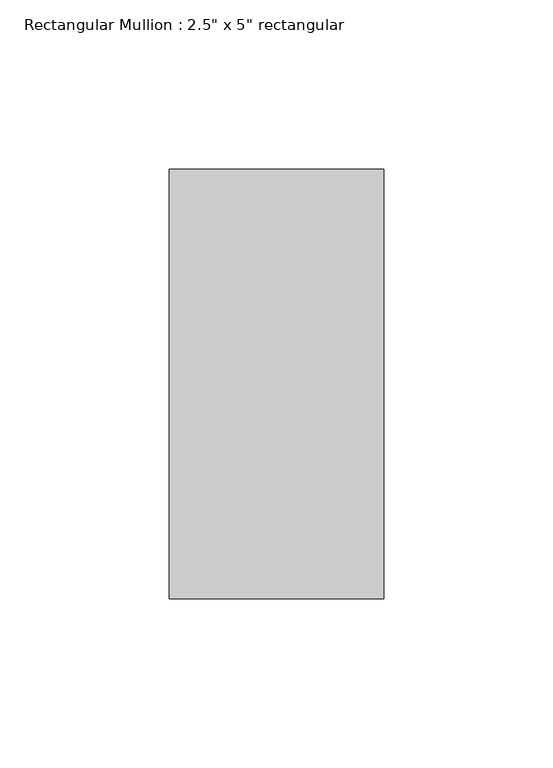
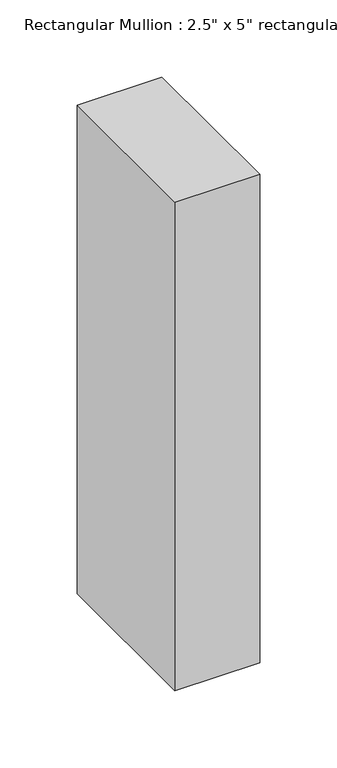
"""IFC4 building model written with IfcOpenShell, lengths in millimetres: member geometry."""

from ifc_helpers import new_model, si_unit, frame, origin, place, context, project, spatial, polyline, outline, extrude, source, transform, mapped, element, save


def member_dffdf235(model_context):
    return source(origin(), model_context, "Body", "SweptSolid", [
        extrude(outline(polyline([(0.0, 63.5), (0.0, -63.5), (-63.5, -63.5), (-63.5, 63.5), (0.0, 63.5)])), frame((0.0, 0.0, -387.35), z_axis=(0.0, 0.0, 1.0), x_axis=(1.0, 0.0, 0.0)), (0.0, 0.0, 1.0), 387.35),
    ])


if __name__ == "__main__":
    model = new_model("IFC4")
    model_context = context("Model", 3, world=origin())
    ifc_project = project(units=[si_unit("LENGTHUNIT", "METRE", prefix="MILLI")], contexts=[model_context])
    site = spatial("IfcSite", under=ifc_project)
    building = spatial("IfcBuilding", under=site)
    placement = place(None, origin())
    member_shape = member_dffdf235(model_context)
    element("IfcMember", 1, ObjectType="Rectangular Mullion : 2.5\" x 5\" rectangular", at=placement, inside=building, context=model_context, shape_type="MappedRepresentation", body=[
        mapped(member_shape, transform((0.0, 0.0, 0.0), x_axis=(1.0, 0.0, 0.0), y_axis=(0.0, 1.0, 0.0), z_axis=(0.0, 0.0, 1.0))),
    ])
    save(model, "model.ifc")

# Revit data of these elements
# Type "Rectangular Mullion : 2.5\" x 5\" rectangular"
#   built-in parameter 1007304 = 0.416667 (stored number, unit not read)
#   built-in parameter 1007301 = 0.104167 (stored number, unit not read)
#   built-in parameter 1007300 = 0.104167 (stored number, unit not read)
# Element 1 (IfcMember, "Rectangular Mullion : 2.5\" x 5\" rectangular")
#   Materials on its faces: "Aluminum"
# Materials
#   "Aluminum": class "Metal", colour RGB 247 247 247, transparency 0, Description = "Aluminum 6061", Cost = 0
